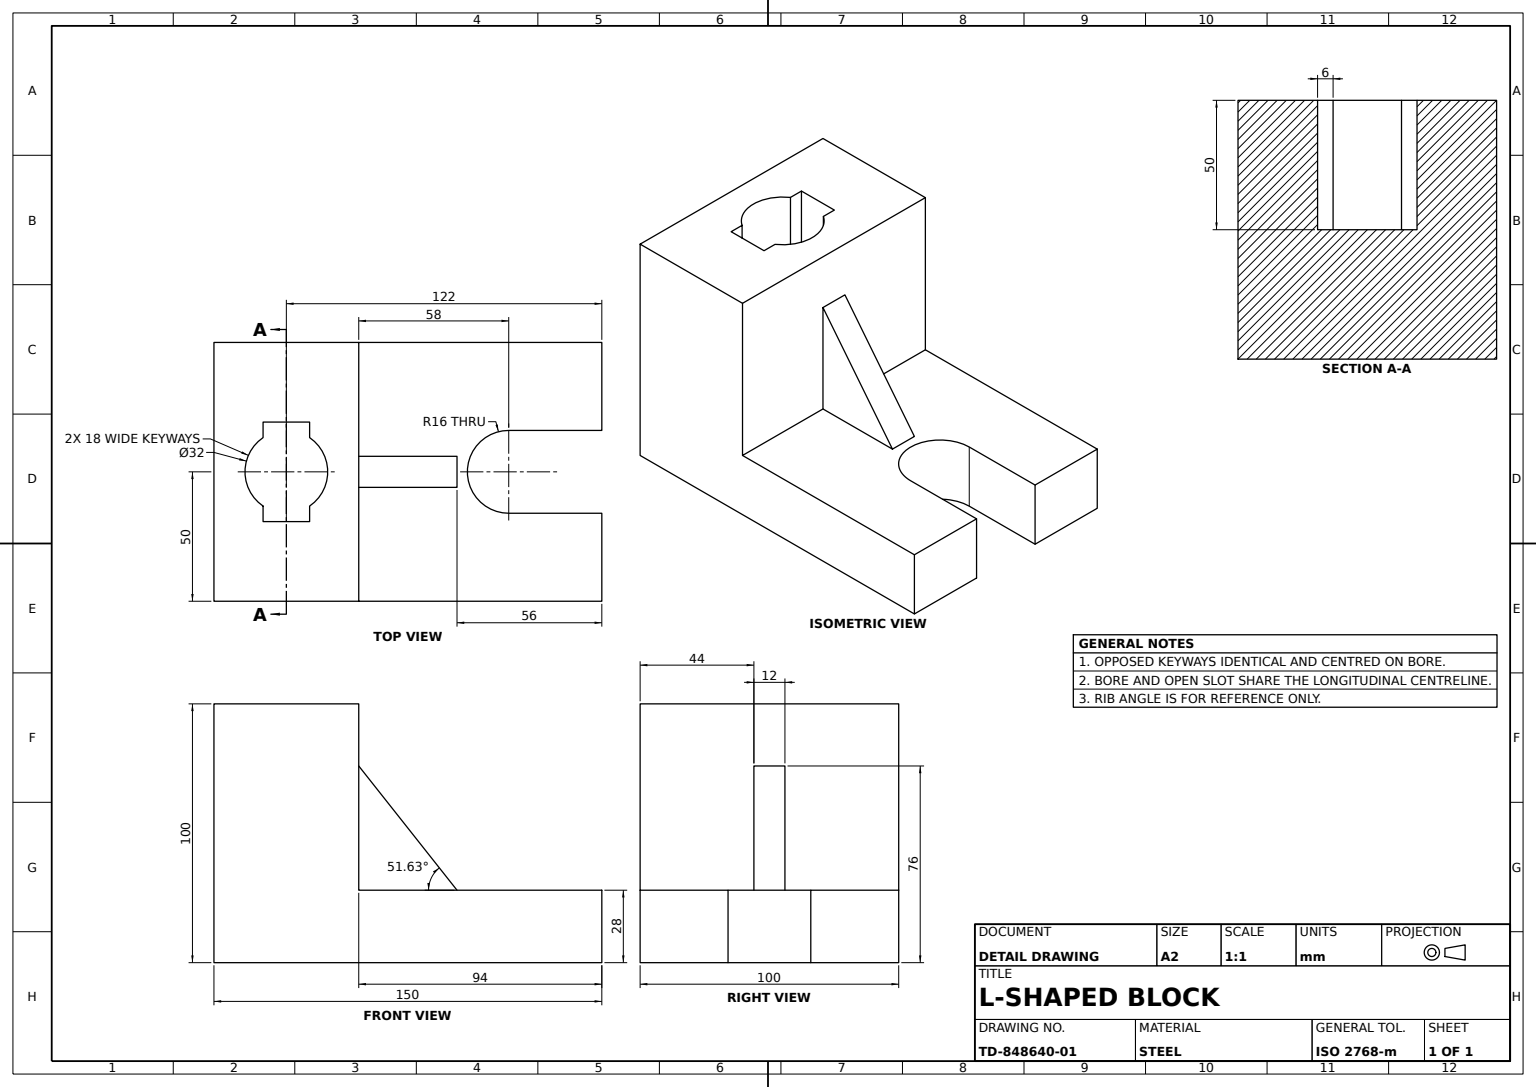
from build123d import *

# Parameters (mm, degrees)
L_BLOCK_BASE_DEPTH      = 100
KEYED_BORE_CUT_DEPTH    = 50
STEP_BOSS_DEPTH         = 60
STEP_CUT_DEPTH          = 44
STEP_RELIEF_CUT_DEPTH   = 4
LOW_STEP_SLOT_CUT_DEPTH = 28


with BuildPart() as part:
    # L-Block Profile Sketch → L-Block Base (new body)
    with BuildSketch(Plane.XY):
        Polygon((0, 0), (150, 0), (150, 100), (94, 100), (94, 28), (0, 28), align=None)
    extrude(amount=L_BLOCK_BASE_DEPTH)

    # Keyed Bore Sketch → Keyed Bore Cut (cut)
    with BuildSketch(Plane(origin=(0, 100, 0), x_dir=(1, 0, 0), z_dir=(0, 1, 0))):
        with BuildLine():
            Line((113, -69.228756555), (131, -69.228756555))
            Line((131, -69.228756555), (131, -63.228756555))
            ThreePointArc((131, -63.228756555), (138, -50), (131, -36.771243445))
            Line((131, -36.771243445), (131, -30.771243445))
            Line((131, -30.771243445), (113, -30.771243445))
            Line((113, -30.771243445), (113, -36.771243445))
            ThreePointArc((113, -36.771243445), (106, -50), (113, -63.228756555))
            Line((113, -63.228756555), (113, -69.228756555))
        make_face()
    extrude(amount=-KEYED_BORE_CUT_DEPTH, mode=Mode.SUBTRACT)

    # Step Boss Sketch → Step Boss (add)
    with BuildSketch(Plane.XY.offset(100)):
        Polygon((94, 28), (94, 76), (56, 28), align=None)
    extrude(amount=-STEP_BOSS_DEPTH)

    # Step Cut Sketch → Step Cut (cut)
    with BuildSketch(Plane.XY.offset(100)):
        Polygon((94, 76), (94, 28), (56, 28), align=None)
    extrude(amount=-STEP_CUT_DEPTH, mode=Mode.SUBTRACT)

    # Step Relief Sketch → Step Relief Cut (cut)
    with BuildSketch(Plane(origin=(0, 0, 40), x_dir=(-1, 0, 0), z_dir=(0, 0, -1))):
        Polygon((-94, 76), (-94, 28), (-56, 28), align=None)
    extrude(amount=-STEP_RELIEF_CUT_DEPTH, mode=Mode.SUBTRACT)

    # Low Step Slot Sketch → Low Step Slot Cut (cut)
    with BuildSketch(Plane(origin=(0, 28, 0), x_dir=(1, 0, 0), z_dir=(0, 1, 0))):
        with BuildLine():
            Line((0, -34), (0, -66))
            Line((0, -66), (36, -66))
            ThreePointArc((36, -66), (52, -50), (36, -34))
            Line((36, -34), (0, -34))
        make_face()
    extrude(amount=-LOW_STEP_SLOT_CUT_DEPTH, mode=Mode.SUBTRACT)


solid = part.part
